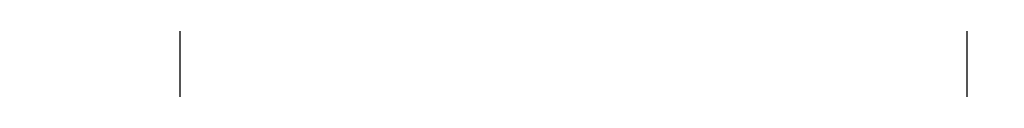
# Model space of a CAD drawing. Units: inches. Extents: x 2091 to 2899, y 967 to 2217.
# Tile 22 of 256: x 2351 to 2390, y 1088 to 1090. Entities that reach past the tile are written whole.
import ezdxf

# ---------------------------------------------------------------- set-up
doc = ezdxf.new("R2010")
doc.units = ezdxf.units.IN
doc.layers.add('A-ANNO-DIMS', color=2, linetype='Continuous', lineweight=18)
doc.styles.get("Standard").update_dxf_attribs({"font": 'arial.ttf'})
doc.dimstyles.new('ISO-25', dxfattribs={"dimtxt": 4, "dimasz": 4, "dimexe": 1.25, "dimexo": 0.625, "dimtad": 1, "dimdec": 0, "dimlunit": 3, "dimtxsty": 'Standard', "dimcen": 2.5, "dimadec": 0, "dimazin": 0, "dimtfac": 1, "dimtdec": 0, "dimtmove": 0, "dimatfit": 3, "dimfxl": 1, "dimarcsym": 0})

# ---------------------------------------------------------------- blocks, each defined once
blk = doc.blocks.new('*D68')
at = {"layer": 'A-ANNO-DIMS', "color": 0, "lineweight": -2, "transparency": 16777216}
for p, q in [((2317.144, 1535.794), (2317.144, 969.464)), ((2459.384, 1535.794), (2459.384, 969.464)), ((2321.144, 970.714), (2455.384, 970.714))]:
    blk.add_line(p, q, dxfattribs=at)
at = {"layer": 'A-ANNO-DIMS', "color": 0, "transparency": 16777216}
for points in [[(2321.144, 971.381), (2321.144, 970.048), (2317.144, 970.714)], [(2455.384, 971.381), (2455.384, 970.048), (2459.384, 970.714)]]:
    blk.add_solid(points, dxfattribs=at)
at = {"layer": 'Defpoints', "color": 0, "transparency": 16777216}
for p in [(2317.144, 1536.419), (2459.384, 1536.419), (2459.384, 970.714)]:
    blk.add_point(p, dxfattribs=at)
at = {"layer": 'A-ANNO-DIMS', "color": 0, "transparency": 16777216, "insert": (2388.264, 973.382), "char_height": 4, "attachment_point": 5}
blk.add_mtext('11\'-10"', dxfattribs=at)
blk = doc.blocks.new('*D71')
at = {"layer": 'A-ANNO-DIMS', "color": 0, "lineweight": -2, "transparency": 16777216}
for p, q in [((2212.144, 1351.294), (2212.144, 969.464)), ((2452.144, 1351.294), (2452.144, 969.464)), ((2216.144, 970.714), (2448.144, 970.714))]:
    blk.add_line(p, q, dxfattribs=at)
at = {"layer": 'A-ANNO-DIMS', "color": 0, "transparency": 16777216}
for points in [[(2216.144, 971.381), (2216.144, 970.048), (2212.144, 970.714)], [(2448.144, 971.381), (2448.144, 970.048), (2452.144, 970.714)]]:
    blk.add_solid(points, dxfattribs=at)
at = {"layer": 'Defpoints', "color": 0, "transparency": 16777216}
for p in [(2212.144, 1351.919), (2452.144, 1351.919), (2452.144, 970.714)]:
    blk.add_point(p, dxfattribs=at)
at = {"layer": 'A-ANNO-DIMS', "color": 0, "transparency": 16777216, "insert": (2332.144, 973.382), "char_height": 4, "attachment_point": 5}
blk.add_mtext('20\'-0"', dxfattribs=at)
blk = doc.blocks.new('*D82')
at = {"layer": 'A-ANNO-DIMS', "color": 0, "lineweight": -2, "transparency": 16777216}
for p, q in [((2357.434, 1549.361), (2357.434, 969.464)), ((2388.969, 1549.361), (2388.969, 969.464)), ((2361.434, 970.714), (2384.969, 970.714))]:
    blk.add_line(p, q, dxfattribs=at)
at = {"layer": 'A-ANNO-DIMS', "color": 0, "transparency": 16777216}
for points in [[(2361.434, 971.381), (2361.434, 970.048), (2357.434, 970.714)], [(2384.969, 971.381), (2384.969, 970.048), (2388.969, 970.714)]]:
    blk.add_solid(points, dxfattribs=at)
at = {"layer": 'Defpoints', "color": 0, "transparency": 16777216}
for p in [(2357.434, 1549.986), (2388.969, 1549.986), (2388.969, 970.714)]:
    blk.add_point(p, dxfattribs=at)
at = {"layer": 'A-ANNO-DIMS', "color": 0, "transparency": 16777216, "insert": (2373.202, 973.408), "char_height": 4, "attachment_point": 5}
blk.add_mtext('2\'-7 1/2"', dxfattribs=at)

msp = doc.modelspace()

# ---------------------------------------------------------------- dimensions: what is measured, and where the dimension line sits
at = {"layer": 'A-ANNO-DIMS'}
for base, p1, p2, picture, middle in [((2388.969, 970.714), (2357.434, 1549.986), (2388.969, 1549.986), '*D82', (2373.202, 973.408)), ((2459.384, 970.714), (2317.144, 1536.419), (2459.384, 1536.419), '*D68', (2388.264, 973.382)), ((2452.144, 970.714), (2212.144, 1351.919), (2452.144, 1351.919), '*D71', (2332.144, 973.382))]:
    dim = msp.add_linear_dim(base=base, p1=p1, p2=p2, dimstyle='ISO-25', override={"dimdec": 1, "dimlfac": 1, "dimrnd": 0, "dimzin": 1, "dimdsep": 46, "dimlunit": 4, "dimfrac": 2}, dxfattribs=at)
    dim.commit()
    dim.dimension.update_dxf_attribs({"geometry": picture, "text_midpoint": middle})

doc.saveas('drawing.dxf')
